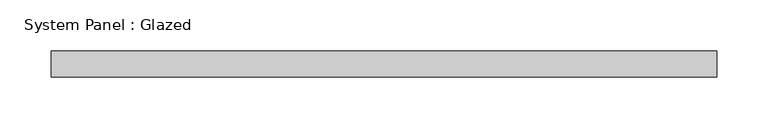
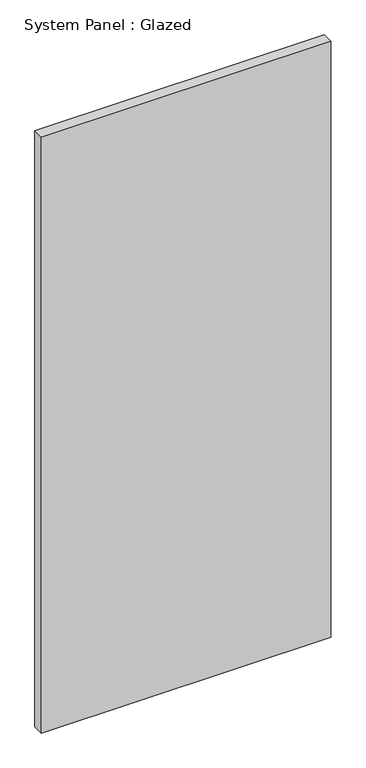
"""IFC4 building model written with IfcOpenShell, lengths in millimetres: plate geometry, System Panel : Glazed."""

from ifc_helpers import new_model, si_unit, origin, origin_with_axes, place, context, project, spatial, polyline, outline, extrude, source, transform, mapped, element, save


def system_panel_glazed_f5702331(model_context):
    return source(origin(), model_context, "Body", "SweptSolid", [
        extrude(outline(polyline([(323.85, 19.05), (-323.85, 19.05), (-323.85, 44.45), (323.85, 44.45), (323.85, 19.05)])), origin_with_axes(), (0.0, 0.0, 1.0), 1411.1940157),
    ])


if __name__ == "__main__":
    model = new_model("IFC4")
    model_context = context("Model", 3, world=origin())
    ifc_project = project(units=[si_unit("LENGTHUNIT", "METRE", prefix="MILLI")], contexts=[model_context])
    site = spatial("IfcSite", under=ifc_project)
    building = spatial("IfcBuilding", under=site)
    placement = place(None, origin())
    system_panel_glazed_shape = system_panel_glazed_f5702331(model_context)
    element("IfcPlate", 1, ObjectType="System Panel : Glazed", at=placement, inside=building, context=model_context, shape_type="MappedRepresentation", body=[
        mapped(system_panel_glazed_shape, transform((0.0, 0.0, 0.0), x_axis=(1.0, 0.0, 0.0), y_axis=(0.0, 1.0, 0.0), z_axis=(0.0, 0.0, 1.0))),
    ])
    save(model, "model.ifc")

# Revit data of these elements
# Type "System Panel : Glazed"
#   Construction Type Id = "GSP4R"
#   Analytic Construction = "1/8 in Pilkington single glazing"
#   Visual Light Transmittance = 0.9
#   Solar Heat Gain Coefficient = 0.86
#   Heat Transfer Coefficient (U) = 1.18115 BTU/(h·ft²·°F)
#   Define Thermal Properties by = 1
# Element 1 (IfcPlate, "System Panel : Glazed")
#   Materials on its faces: "Glass"
# Materials
#   "Glass": class "Glass", colour RGB 0 128 192, transparency 0.75, Description = "Soda Lime Glass", Cost = 0
